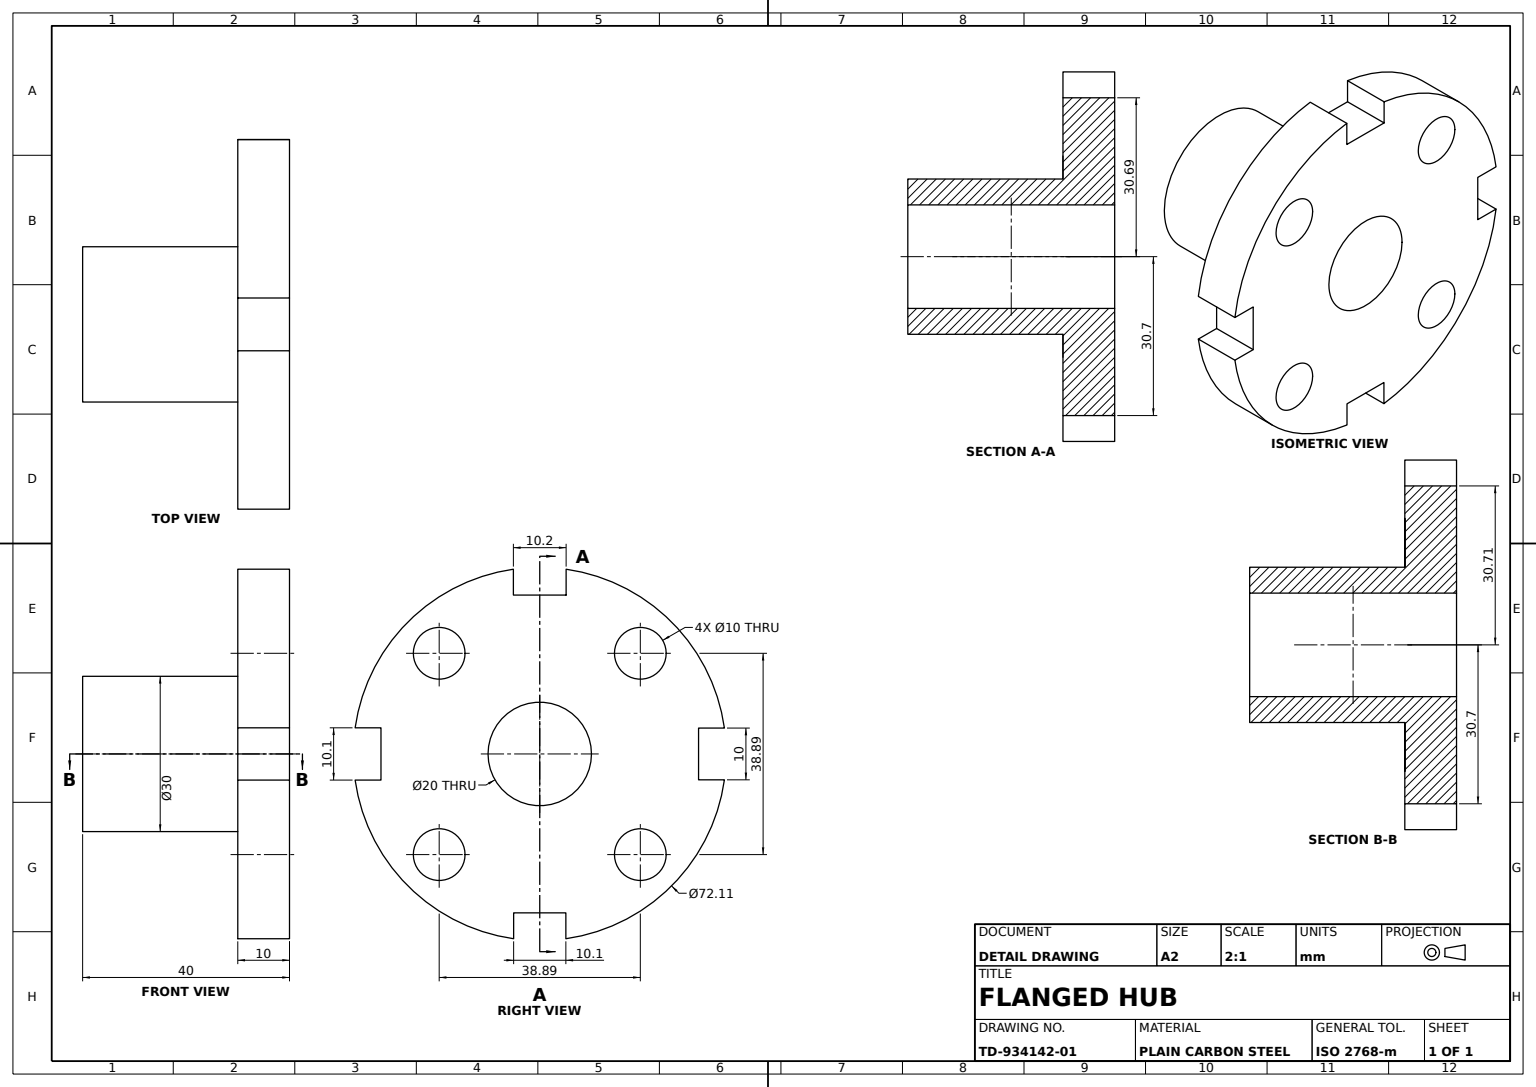
SolidWorks part; units mm, degrees
material "Plain Carbon Steel"
ref_plane "Front Plane" through (0, 0, 0) normal (0, 0, 1) x (1, 0, 0)
ref_plane "Top Plane" through (0, 0, 0) normal (0, 1, 0) x (1, 0, 0)
ref_plane "Right Plane" through (0, 0, 0) normal (1, 0, 0) x (0, 0, -1)
sketch "Flange Profile Sketch" plane through (0, 0, 0) normal (0, 0, 1) x (1, 0, 0)
  line L1 (0, 30.6931) -> (5.099, 30.6931)
  line L2 (5.099, 30.6931) -> (5.099, 35.6931)
  line L3 (0, 30.6931) -> (-5.099, 30.6931)
  line L4 (-5.099, 30.6931) -> (-5.099, 35.6931)
  line L6 (0, -30.7003) -> (5.0488, -30.7003)
  line L7 (5.0488, -30.7003) -> (5.0488, -35.7003)
  line L8 (0, -30.7003) -> (-5.0488, -30.7003)
  line L9 (-5.0488, -30.7003) -> (-5.0488, -35.7003)
  line L11 (30.7003, 0) -> (30.7003, 5.0488)
  line L12 (30.7003, 5.0488) -> (35.7003, 5.0488)
  line L13 (30.7003, 0) -> (30.7003, -5.0488)
  line L14 (30.7003, -5.0488) -> (35.7003, -5.0488)
  line L16 (-30.7071, 0) -> (-30.7071, 5)
  line L17 (-30.7071, 5) -> (-35.7071, 5)
  line L18 (-30.7071, 0) -> (-30.7071, -5)
  line L19 (-30.7071, -5) -> (-35.7071, -5)
  arc A0 (-5.099, 35.6931) -> (-35.7071, 5) centre (0, 0) ccw
  arc A1 (35.7003, 5.0488) -> (5.099, 35.6931) centre (0, 0) ccw
  arc A2 (-35.7071, -5) -> (-5.0488, -35.7003) centre (0, 0) ccw
  arc A3 (5.0488, -35.7003) -> (35.7003, -5.0488) centre (0, 0) ccw
  dimension "D1" = 72.111
  dimension "D2" = 36.0555
  dimension "D3" = 25.6081
  dimension "D4" = 25.6584
  dimension "D5" = 30.7071
extrude "Flange Plate" add sketch "Flange Profile Sketch" along normal blind 10
sketch "Mounting Holes Sketch" plane through (0, 0, 10) normal (0, 0, 1) x (1, 0, 0)
  line L0 (-30.7071, 5) -> (-30.7071, -5) construction
  line L1 (5.099, 30.6931) -> (-5.099, 30.6931) construction
  circle A1 centre (19.4454, 19.4454) radius 5
  circle A2 centre (19.4454, -19.4454) radius 5
  circle A3 centre (-19.4454, -19.4454) radius 5
  circle A4 centre (-19.4454, 19.4454) radius 5
  dimension "D3" = 50.1526
  dimension "D4" = 10
  dimension "D5" = 10
  dimension "D6" = 10
  dimension "D7" = 10
  dimension "D1" = 10
  dimension "D2" = 11.2617
  dimension "D8" = 11.2477
  dimension "D9" = 50.1386
extrude "Mounting Holes 4xØ10" cut sketch "Mounting Holes Sketch" against normal blind 10
sketch "Hub Sketch" plane through (0, 0, 10) normal (0, 0, 1) x (1, 0, 0)
  circle A0 centre (0, 0) radius 15
  dimension "D1" = 30
  dimension "D2" = 30
extrude "Hub Ø30" add sketch "Hub Sketch" along normal blind 30
sketch "Hub Bore Sketch" plane through (0, 0, 40) normal (0, 0, 1) x (1, 0, 0)
  circle A0 centre (0, 0) radius 10
  dimension "D1" = 20
  dimension "D2" = 20
extrude "Hub Bore Ø20" cut sketch "Hub Bore Sketch" against normal blind 30
sketch "Flange Bore Sketch" plane through (0, 0, 10) normal (0, 0, 1) x (1, 0, 0)
  circle A0 centre (0, 0) radius 10
  dimension "D1" = 20
  dimension "D2" = 20
extrude "Flange Bore Ø20" cut sketch "Flange Bore Sketch" against normal blind 30
